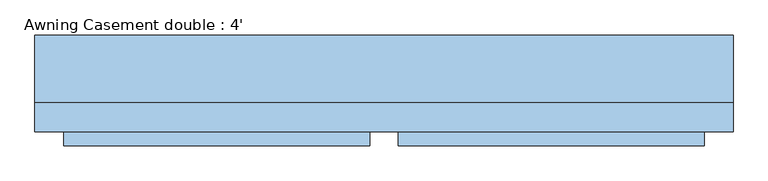
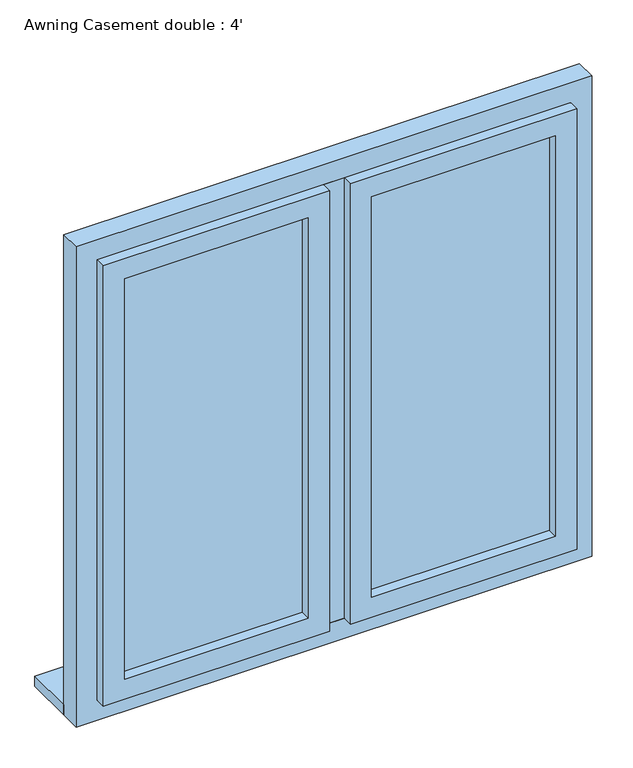
"""IFC4 building model written with IfcOpenShell, lengths in millimetres: window geometry, Awning Casement double : 4'."""

from ifc_helpers import new_model, si_unit, frame, origin, place, context, project, spatial, polyline, outline, extrude, source, transform, mapped, element, save


def awning_casement_double_4_37d249be(model_context):
    return source(origin(), model_context, "Body", "SweptSolid", [
        extrude(outline(polyline([(2000.0, 609.6), (2000.0, -609.6), (800.0, -609.6), (800.0, 609.6), (2000.0, 609.6)]), holes=[polyline([(1950.0, 559.6), (850.0, 559.6), (850.0, -559.6), (1950.0, -559.6), (1950.0, 559.6)])]), frame((0.0, -24.5, 0.0), z_axis=(0.0, 1.0, 0.0), x_axis=(0.0, 0.0, 1.0)), (0.0, 0.0, 1.0), 50.0),
        extrude(outline(polyline([(1950.0, -25.0), (1950.0, -559.6), (850.0, -559.6), (850.0, -25.0), (1950.0, -25.0)]), holes=[polyline([(1900.0, -75.0), (900.0, -75.0), (900.0, -509.6), (1900.0, -509.6), (1900.0, -75.0)])]), frame((0.0, -49.5, 0.0), z_axis=(0.0, 1.0, 0.0), x_axis=(0.0, 0.0, 1.0)), (0.0, 0.0, 1.0), 49.5),
        extrude(outline(polyline([(1950.0, 559.6), (1950.0, 25.0), (850.0, 25.0), (850.0, 559.6), (1950.0, 559.6)]), holes=[polyline([(1900.0, 509.6), (900.0, 509.6), (900.0, 75.0), (1900.0, 75.0), (1900.0, 509.6)])]), frame((0.0, -49.5, 0.0), z_axis=(0.0, 1.0, 0.0), x_axis=(0.0, 0.0, 1.0)), (0.0, 0.0, 1.0), 49.5),
        extrude(outline(polyline([(25.0, -24.5), (-25.0, -24.5), (-25.0, 25.5), (25.0, 25.5), (25.0, -24.5)])), frame((0.0, 0.0, 850.0), z_axis=(0.0, 0.0, 1.0), x_axis=(1.0, 0.0, 0.0)), (0.0, 0.0, 1.0), 1100.0),
        extrude(outline(polyline([(-75.0, -25.5), (-509.6, -25.5), (-509.6, -24.5), (-75.0, -24.5), (-75.0, -25.5)])), frame((0.0, 0.0, 900.0), z_axis=(0.0, 0.0, 1.0), x_axis=(1.0, 0.0, 0.0)), (0.0, 0.0, 1.0), 1000.0),
        extrude(outline(polyline([(509.6, -25.5), (75.0, -25.5), (75.0, -24.5), (509.6, -24.5), (509.6, -25.5)])), frame((0.0, 0.0, 900.0), z_axis=(0.0, 0.0, 1.0), x_axis=(1.0, 0.0, 0.0)), (0.0, 0.0, 1.0), 1000.0),
        extrude(outline(polyline([(609.6, 25.5), (-609.6, 25.5), (-609.6, 144.3), (609.6, 144.3), (609.6, 25.5)])), frame((0.0, 0.0, 800.0), z_axis=(0.0, 0.0, 1.0), x_axis=(1.0, 0.0, 0.0)), (0.0, 0.0, 1.0), 25.0),
    ])


if __name__ == "__main__":
    model = new_model("IFC4")
    model_context = context("Model", 3, world=origin())
    ifc_project = project(units=[si_unit("LENGTHUNIT", "METRE", prefix="MILLI")], contexts=[model_context])
    site = spatial("IfcSite", under=ifc_project)
    building = spatial("IfcBuilding", under=site)
    placement = place(None, origin())
    awning_casement_double_4_shape = awning_casement_double_4_37d249be(model_context)
    element("IfcWindow", 1, ObjectType="Awning Casement double : 4'", at=placement, inside=building, context=model_context, shape_type="MappedRepresentation", body=[
        mapped(awning_casement_double_4_shape, transform((0.0, 0.0, 0.0), x_axis=(1.0, 0.0, 0.0), y_axis=(0.0, 1.0, 0.0), z_axis=(0.0, 0.0, 1.0))),
    ])
    save(model, "model.ifc")

# Revit data of these elements
# Type "Awning Casement double : 4'"
#   Type Mark = "21"
#   Operation = "DoublePanelVertical"
#   Keynote = "L10/210"
#   Height = 3' - 11.24409"
#   Default Sill Height = 2' - 7.49606"
#   Width = 4' - 0"
#   Wall Closure = (empty or 0)
# Element 1 (IfcWindow, "Awning Casement double : 4'")
#   Materials on its faces: "Default Frame", "Glass", "Default Sill"
# Materials
#   "Default Frame": colour RGB 193 168 117, transparency 0
#   "Glass": class "Glass", colour RGB 0 128 192, transparency 0.75, Description = "Soda Lime Glass", Cost = 0
#   "Default Sill": colour RGB 188 165 158, transparency 0
